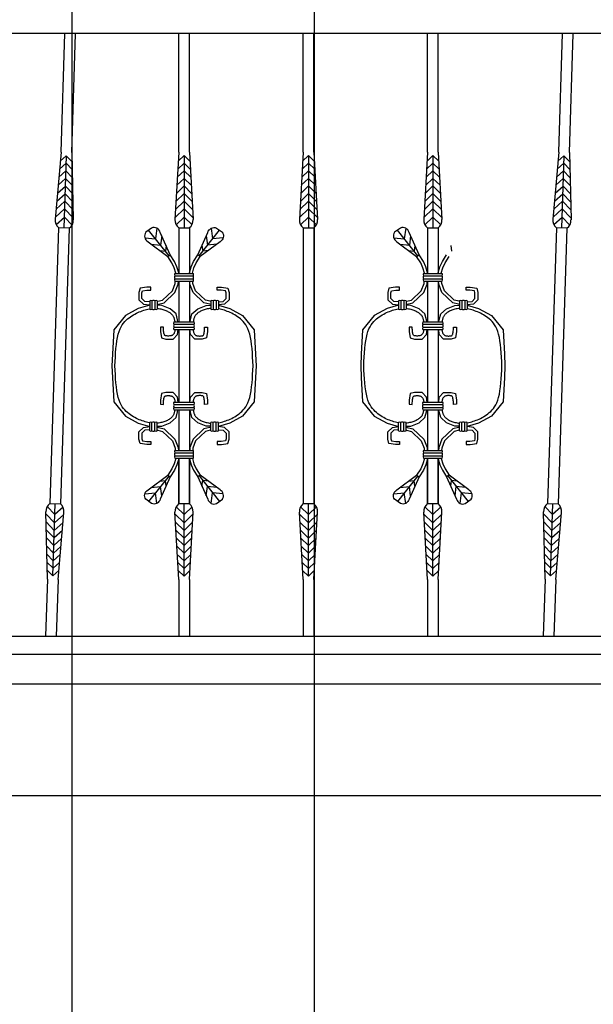
# Model space of a CAD drawing. Units: inches. Extents: x 2278 to 7495, y -71 to 1198.
# Tile 11 of 44: x 4907 to 4938, y 107 to 160. Entities that reach past the tile are written whole.
import ezdxf

# ---------------------------------------------------------------- set-up
doc = ezdxf.new("R2010")
doc.units = ezdxf.units.IN
doc.header["$MEASUREMENT"] = 0
doc.layers.add('A-ANNO-DIMS', color=2, linetype='Continuous', lineweight=18)
doc.layers.add('A-ELEV', color=7, linetype='Continuous', lineweight=25)
doc.styles.get("Standard").update_dxf_attribs({"font": 'arial.ttf'})
doc.dimstyles.get("Standard").update_dxf_attribs({"dimtxt": 6, "dimasz": 3, "dimexe": 0.18, "dimexo": 0.0625, "dimgap": 0.09, "dimtad": 0, "dimtih": 1, "dimtoh": 1, "dimdec": 0, "dimzin": 0, "dimdsep": 46, "dimlunit": 3, "dimtxsty": 'Standard', "dimblk": 'ARCHTICK', "dimcen": 0.09, "dimadec": 0, "dimazin": 0, "dimtfac": 1, "dimtdec": 0, "dimtofl": 0, "dimtmove": 0, "dimatfit": 3, "dimfxl": 1, "dimtolj": 1, "dimtzin": 0, "dimarcsym": 0})

# ---------------------------------------------------------------- blocks, each defined once
blk = doc.blocks.new('BALUSTER-ORNATE-C')
for p, q in [((3.585, 26.003), (3.585, 32.384)), ((4.155, 26.003), (4.155, 32.38)), ((3.585, 26.003), (3.383, 22.393)), ((4.155, 26.003), (4.357, 22.393)), ((3.533, 25.084), (3.87, 25.41)), ((3.557, 25.516), (3.87, 25.818)), ((3.87, 25.818), (3.87, 21.929)), ((4.182, 25.516), (3.87, 25.818)), ((4.206, 25.084), (3.87, 25.41)), ((3.509, 24.653), (3.87, 25.001)), ((4.231, 24.653), (3.87, 25.001)), ((3.485, 24.221), (3.87, 24.593)), ((4.255, 24.221), (3.87, 24.593)), ((3.461, 23.79), (3.87, 24.185)), ((4.279, 23.79), (3.87, 24.185)), ((3.412, 22.927), (3.87, 23.369)), ((3.437, 23.358), (3.87, 23.777)), ((4.303, 23.358), (3.87, 23.777)), ((4.327, 22.927), (3.87, 23.369)), ((3.388, 22.495), (3.87, 22.961)), ((4.351, 22.495), (3.87, 22.961)), ((3.441, 22.106), (3.87, 22.52)), ((4.298, 22.106), (3.87, 22.52)), ((3.063, 20.442), (1.97, 21.814)), ((2.412, 21.914), (2.338, 21.352)), ((3.585, 21.929), (3.585, 19.485)), ((4.155, 21.929), (3.585, 21.929)), ((4.155, 21.929), (4.155, 19.485)), ((4.677, 20.442), (5.769, 21.814)), ((5.328, 21.914), (5.401, 21.352)), ((1.774, 21.406), (2.338, 21.352)), ((2.678, 21.507), (2.613, 21.007)), ((5.061, 21.507), (5.127, 21.007)), ((5.966, 21.406), (5.401, 21.352)), ((2.111, 21.055), (2.613, 21.007)), ((2.562, 20.717), (2.867, 20.688)), ((2.907, 20.992), (2.867, 20.688)), ((4.833, 20.992), (4.872, 20.688)), ((5.177, 20.717), (4.872, 20.688)), ((5.629, 21.055), (5.127, 21.007)), ((3.37, 19.485), (4.37, 19.485)), ((3.37, 19.363), (4.37, 19.363)), ((3.37, 19.2), (4.37, 19.2)), ((3.37, 19.077), (4.37, 19.077)), ((3.585, 19.077), (3.585, 16.887)), ((4.155, 19.077), (4.155, 16.887)), ((2.026, 18.021), (2.026, 17.565)), ((2.148, 18.021), (2.148, 17.565)), ((2.311, 18.021), (2.311, 17.565)), ((2.433, 18.021), (2.433, 17.565)), ((5.306, 18.021), (5.306, 17.565)), ((5.428, 18.021), (5.428, 17.565)), ((5.591, 18.021), (5.591, 17.565)), ((5.714, 18.021), (5.714, 17.565)), ((3.329, 16.887), (4.411, 16.887)), ((3.329, 16.764), (4.411, 16.764)), ((3.329, 16.601), (4.411, 16.601)), ((3.329, 16.479), (4.411, 16.479)), ((3.585, 16.479), (3.585, 12.578)), ((4.155, 16.479), (4.155, 12.578)), ((3.329, 12.578), (4.411, 12.578)), ((3.329, 12.456), (4.411, 12.456)), ((3.329, 12.293), (4.411, 12.293)), ((3.329, 12.171), (4.411, 12.171)), ((3.585, 12.171), (3.585, 9.98)), ((4.155, 12.171), (4.155, 9.98)), ((2.026, 11.037), (2.026, 11.493)), ((2.148, 11.037), (2.148, 11.493)), ((2.311, 11.037), (2.311, 11.493)), ((2.433, 11.037), (2.433, 11.493)), ((5.306, 11.037), (5.306, 11.493)), ((5.428, 11.037), (5.428, 11.493)), ((5.591, 11.037), (5.591, 11.493)), ((5.714, 11.037), (5.714, 11.493)), ((3.37, 9.98), (4.37, 9.98)), ((3.37, 9.858), (4.37, 9.858)), ((3.37, 9.695), (4.37, 9.695)), ((3.37, 9.573), (4.37, 9.573)), ((3.585, 9.573), (3.585, 7.095)), ((3.585, 7.095), (3.585, 9.573)), ((4.155, 9.573), (4.155, 7.095)), ((4.155, 7.095), (4.155, 9.573)), ((3.063, 8.615), (1.97, 7.244)), ((4.677, 8.615), (5.769, 7.244)), ((2.111, 8.002), (2.613, 8.051)), ((2.562, 8.34), (2.867, 8.37)), ((2.678, 7.551), (2.613, 8.051)), ((2.907, 8.066), (2.867, 8.37)), ((4.833, 8.066), (4.872, 8.37)), ((5.177, 8.34), (4.872, 8.37)), ((5.061, 7.551), (5.127, 8.051)), ((5.629, 8.002), (5.127, 8.051)), ((1.774, 7.651), (2.338, 7.706)), ((2.412, 7.143), (2.338, 7.706)), ((5.328, 7.143), (5.401, 7.706)), ((5.966, 7.651), (5.401, 7.706)), ((3.441, 6.952), (3.87, 6.538)), ((3.585, 7.128), (4.155, 7.128)), ((3.87, 3.24), (3.87, 7.128)), ((4.298, 6.952), (3.87, 6.538)), ((3.585, 3.055), (3.383, 6.664)), ((3.388, 6.562), (3.87, 6.097)), ((4.351, 6.562), (3.87, 6.097)), ((4.155, 3.055), (4.357, 6.664)), ((3.412, 6.131), (3.87, 5.689)), ((4.327, 6.131), (3.87, 5.689)), ((3.437, 5.699), (3.87, 5.28)), ((4.303, 5.699), (3.87, 5.28)), ((3.461, 5.268), (3.87, 4.872)), ((3.485, 4.836), (3.87, 4.464)), ((4.279, 5.268), (3.87, 4.872)), ((4.255, 4.836), (3.87, 4.464)), ((3.509, 4.405), (3.87, 4.056)), ((4.231, 4.405), (3.87, 4.056)), ((3.533, 3.973), (3.87, 3.648)), ((4.206, 3.973), (3.87, 3.648)), ((3.557, 3.542), (3.87, 3.24)), ((4.182, 3.542), (3.87, 3.24)), ((3.585, 3.055), (3.585, 0)), ((4.155, 3.055), (4.155, 0))]:
    blk.add_line(p, q)
for points in [[(3.131, 20.487), (2.594, 21.696, 0.435351), (2.128, 21.929), (1.813, 21.699, 0.435351), (1.936, 21.192), (2.995, 20.398)], [(4.608, 20.487), (5.145, 21.696, -0.435351), (5.612, 21.929), (5.927, 21.699, -0.435351), (5.804, 21.192), (4.745, 20.398)], [(3.131, 8.571), (2.594, 7.362, -0.435351), (2.128, 7.128), (1.813, 7.359, -0.435351), (1.936, 7.866), (2.995, 8.66)], [(4.608, 8.571), (5.145, 7.362, 0.435351), (5.612, 7.128), (5.927, 7.359, 0.435351), (5.804, 7.866), (4.745, 8.66)]]:
    blk.add_lwpolyline(points, format="xyb", close=True)
for points in [[(3.42, 19.485), (3.421, 19.506), (3.336, 19.795), (3.216, 20.057), (2.995, 20.398)], [(3.583, 19.485), (3.585, 19.526), (3.489, 19.852), (3.359, 20.135), (3.131, 20.487)], [(4.157, 19.485), (4.155, 19.526), (4.25, 19.852), (4.38, 20.135), (4.608, 20.487)], [(4.32, 19.485), (4.319, 19.506), (4.403, 19.795), (4.523, 20.057), (4.745, 20.398)], [(2.433, 17.826), (2.492, 17.833), (2.801, 17.915), (3.385, 18.463), (3.557, 18.908), (3.565, 19.077)], [(2.433, 17.99), (2.462, 17.993), (2.719, 18.062), (3.247, 18.557), (3.396, 18.942), (3.402, 19.077)], [(5.306, 17.826), (5.247, 17.833), (4.939, 17.915), (4.355, 18.463), (4.182, 18.908), (4.175, 19.077)], [(5.306, 17.99), (5.278, 17.993), (5.02, 18.062), (4.493, 18.557), (4.344, 18.942), (4.338, 19.077)], [(2.026, 17.961), (1.767, 17.989), (1.612, 18.138), (1.612, 18.447), (1.642, 18.56), (1.879, 18.596), (2.084, 18.596), (2.084, 18.759), (1.866, 18.759), (1.512, 18.705), (1.449, 18.469), (1.449, 18.069), (1.694, 17.833), (2.026, 17.797)], [(5.714, 17.961), (5.973, 17.989), (6.128, 18.138), (6.128, 18.447), (6.098, 18.56), (5.861, 18.596), (5.656, 18.596), (5.656, 18.759), (5.873, 18.759), (6.227, 18.705), (6.291, 18.469), (6.291, 18.069), (6.046, 17.833), (5.714, 17.797)], [(2.026, 17.782), (1.412, 17.603), (0.722, 17.231), (0.095, 16.469), (0.025, 15.162), (0, 14.529), (0.025, 13.895), (0.095, 12.589), (0.722, 11.827), (1.412, 11.455), (2.026, 11.276)], [(0.163, 14.522), (0.173, 14.759), (0.184, 14.995), (0.199, 15.227), (0.217, 15.452), (0.239, 15.667), (0.267, 15.87), (0.3, 16.057), (0.34, 16.227), (0.386, 16.376), (0.438, 16.508), (0.495, 16.624), (0.557, 16.727), (0.623, 16.819), (0.692, 16.9), (0.764, 16.975), (0.839, 17.043), (0.916, 17.105), (0.993, 17.163), (1.071, 17.216), (1.15, 17.265), (1.229, 17.309), (1.309, 17.35), (1.389, 17.388), (1.469, 17.422), (1.548, 17.454), (1.627, 17.484), (1.705, 17.51), (1.782, 17.533), (1.858, 17.553), (1.933, 17.571), (2.007, 17.585), (2.026, 17.587)], [(3.541, 16.887), (3.527, 17.004), (3.446, 17.313), (3.128, 17.594), (2.683, 17.766), (2.433, 17.777)], [(2.433, 17.606), (2.499, 17.6), (2.563, 17.592), (2.624, 17.582), (2.683, 17.57), (2.739, 17.556), (2.792, 17.54), (2.842, 17.522), (2.891, 17.503), (2.937, 17.482), (2.981, 17.46), (3.023, 17.436), (3.064, 17.41), (3.102, 17.384), (3.138, 17.357), (3.171, 17.329), (3.201, 17.301), (3.228, 17.272), (3.251, 17.244), (3.271, 17.217), (3.288, 17.19), (3.303, 17.162), (3.316, 17.134), (3.327, 17.104), (3.337, 17.072), (3.345, 17.038), (3.354, 17.001), (3.361, 16.962), (3.368, 16.922), (3.374, 16.887)], [(4.198, 16.887), (4.212, 17.004), (4.294, 17.313), (4.612, 17.594), (5.057, 17.766), (5.306, 17.777)], [(5.306, 17.606), (5.241, 17.6), (5.177, 17.592), (5.115, 17.582), (5.057, 17.57), (5.001, 17.556), (4.948, 17.54), (4.897, 17.522), (4.849, 17.503), (4.803, 17.482), (4.759, 17.46), (4.716, 17.436), (4.676, 17.41), (4.638, 17.384), (4.602, 17.357), (4.569, 17.329), (4.539, 17.301), (4.512, 17.272), (4.488, 17.244), (4.468, 17.217), (4.451, 17.19), (4.437, 17.162), (4.424, 17.134), (4.413, 17.104), (4.403, 17.072), (4.394, 17.038), (4.386, 17.001), (4.379, 16.962), (4.371, 16.922), (4.366, 16.887)], [(5.714, 17.782), (6.328, 17.603), (7.018, 17.231), (7.644, 16.469), (7.715, 15.162), (7.74, 14.529), (7.715, 13.895), (7.644, 12.589), (7.018, 11.827), (6.328, 11.455), (5.714, 11.276)], [(7.577, 14.522), (7.567, 14.759), (7.555, 14.995), (7.541, 15.227), (7.523, 15.452), (7.501, 15.667), (7.473, 15.87), (7.44, 16.057), (7.4, 16.227), (7.354, 16.376), (7.302, 16.508), (7.244, 16.624), (7.183, 16.727), (7.117, 16.819), (7.048, 16.9), (6.976, 16.975), (6.901, 17.043), (6.824, 17.105), (6.747, 17.163), (6.668, 17.216), (6.59, 17.265), (6.51, 17.309), (6.431, 17.35), (6.351, 17.388), (6.271, 17.422), (6.191, 17.454), (6.113, 17.484), (6.035, 17.51), (5.958, 17.533), (5.882, 17.553), (5.807, 17.571), (5.733, 17.585), (5.714, 17.587)], [(3.388, 16.479), (3.383, 16.441), (3.376, 16.401), (3.368, 16.364), (3.357, 16.329), (3.346, 16.299), (3.333, 16.271), (3.318, 16.247), (3.303, 16.225), (3.286, 16.207), (3.268, 16.19), (3.249, 16.176), (3.228, 16.164), (3.205, 16.154), (3.179, 16.145), (3.149, 16.138), (3.116, 16.133), (3.081, 16.13), (3.045, 16.129), (3.007, 16.129), (2.971, 16.131), (2.936, 16.134), (2.905, 16.137), (2.88, 16.142), (2.863, 16.146), (2.852, 16.151), (2.845, 16.154), (2.84, 16.159), (2.834, 16.166), (2.825, 16.18), (2.814, 16.203), (2.803, 16.237), (2.792, 16.28), (2.783, 16.331), (2.775, 16.388), (2.769, 16.452), (2.766, 16.522), (2.764, 16.599), (2.601, 16.596), (2.601, 16.378), (2.656, 16.024), (2.892, 15.961), (3.291, 15.961), (3.527, 16.206), (3.557, 16.479)], [(4.352, 16.479), (4.357, 16.441), (4.364, 16.401), (4.372, 16.364), (4.382, 16.329), (4.394, 16.299), (4.407, 16.271), (4.421, 16.247), (4.437, 16.225), (4.454, 16.207), (4.472, 16.19), (4.491, 16.176), (4.512, 16.164), (4.534, 16.154), (4.56, 16.145), (4.59, 16.138), (4.623, 16.133), (4.659, 16.13), (4.695, 16.129), (4.732, 16.129), (4.769, 16.131), (4.804, 16.134), (4.835, 16.137), (4.86, 16.142), (4.877, 16.146), (4.888, 16.151), (4.894, 16.154), (4.899, 16.159), (4.906, 16.166), (4.914, 16.18), (4.925, 16.203), (4.937, 16.237), (4.948, 16.28), (4.957, 16.331), (4.965, 16.388), (4.971, 16.452), (4.974, 16.522), (4.975, 16.599), (5.138, 16.596), (5.138, 16.378), (5.084, 16.024), (4.848, 15.961), (4.448, 15.961), (4.212, 16.206), (4.182, 16.479)], [(2.026, 11.47), (2.007, 11.473), (1.933, 11.487), (1.858, 11.504), (1.782, 11.524), (1.705, 11.548), (1.627, 11.574), (1.548, 11.603), (1.469, 11.635), (1.389, 11.67), (1.309, 11.708), (1.229, 11.748), (1.15, 11.793), (1.071, 11.841), (0.993, 11.894), (0.916, 11.952), (0.839, 12.015), (0.764, 12.083), (0.692, 12.157), (0.623, 12.239), (0.557, 12.33), (0.495, 12.433), (0.438, 12.549), (0.386, 12.681), (0.34, 12.831), (0.3, 13), (0.267, 13.188), (0.239, 13.391), (0.217, 13.606), (0.199, 13.831), (0.184, 14.062), (0.173, 14.298), (0.163, 14.536)], [(5.714, 11.47), (5.733, 11.473), (5.807, 11.487), (5.882, 11.504), (5.958, 11.524), (6.035, 11.548), (6.113, 11.574), (6.191, 11.603), (6.271, 11.635), (6.351, 11.67), (6.431, 11.708), (6.51, 11.748), (6.59, 11.793), (6.668, 11.841), (6.747, 11.894), (6.824, 11.952), (6.901, 12.015), (6.976, 12.083), (7.048, 12.157), (7.117, 12.239), (7.183, 12.33), (7.244, 12.433), (7.302, 12.549), (7.354, 12.681), (7.4, 12.831), (7.44, 13), (7.473, 13.188), (7.501, 13.391), (7.523, 13.606), (7.541, 13.831), (7.555, 14.062), (7.567, 14.298), (7.577, 14.536)], [(3.557, 12.578), (3.527, 12.852), (3.291, 13.097), (2.892, 13.097), (2.656, 13.033), (2.601, 12.679), (2.601, 12.462), (2.764, 12.459), (2.766, 12.536), (2.769, 12.605), (2.775, 12.669), (2.783, 12.727), (2.792, 12.778), (2.803, 12.82), (2.814, 12.854), (2.825, 12.878), (2.834, 12.892), (2.84, 12.899), (2.845, 12.903), (2.852, 12.907), (2.863, 12.911), (2.88, 12.916), (2.905, 12.92), (2.936, 12.924), (2.971, 12.927), (3.007, 12.929), (3.045, 12.929), (3.081, 12.928), (3.116, 12.924), (3.149, 12.919), (3.179, 12.912), (3.205, 12.904), (3.228, 12.893), (3.249, 12.881), (3.268, 12.867), (3.286, 12.851), (3.303, 12.832), (3.318, 12.811), (3.333, 12.786), (3.346, 12.759), (3.357, 12.728), (3.368, 12.694), (3.376, 12.656), (3.383, 12.616), (3.388, 12.578)], [(4.182, 12.578), (4.212, 12.852), (4.448, 13.097), (4.848, 13.097), (5.084, 13.033), (5.138, 12.679), (5.138, 12.462), (4.975, 12.459), (4.974, 12.536), (4.971, 12.605), (4.965, 12.669), (4.957, 12.727), (4.948, 12.778), (4.937, 12.82), (4.925, 12.854), (4.914, 12.878), (4.906, 12.892), (4.899, 12.899), (4.894, 12.903), (4.888, 12.907), (4.877, 12.911), (4.86, 12.916), (4.835, 12.92), (4.804, 12.924), (4.769, 12.927), (4.732, 12.929), (4.695, 12.929), (4.659, 12.928), (4.623, 12.924), (4.59, 12.919), (4.56, 12.912), (4.534, 12.904), (4.512, 12.893), (4.491, 12.881), (4.472, 12.867), (4.454, 12.851), (4.437, 12.832), (4.421, 12.811), (4.407, 12.786), (4.394, 12.759), (4.382, 12.728), (4.372, 12.694), (4.364, 12.656), (4.357, 12.616), (4.352, 12.578)], [(3.374, 12.171), (3.368, 12.136), (3.361, 12.095), (3.354, 12.056), (3.345, 12.02), (3.337, 11.986), (3.327, 11.954), (3.316, 11.924), (3.303, 11.895), (3.288, 11.868), (3.271, 11.841), (3.251, 11.813), (3.228, 11.785), (3.201, 11.757), (3.171, 11.729), (3.138, 11.701), (3.102, 11.673), (3.064, 11.647), (3.023, 11.622), (2.981, 11.598), (2.937, 11.576), (2.891, 11.555), (2.842, 11.535), (2.792, 11.518), (2.739, 11.502), (2.683, 11.488), (2.624, 11.476), (2.563, 11.465), (2.499, 11.457), (2.433, 11.451)], [(2.433, 11.28), (2.683, 11.291), (3.128, 11.464), (3.446, 11.745), (3.527, 12.053), (3.541, 12.171)], [(5.306, 11.28), (5.057, 11.291), (4.612, 11.464), (4.294, 11.745), (4.212, 12.053), (4.198, 12.171)], [(4.366, 12.171), (4.371, 12.136), (4.379, 12.095), (4.386, 12.056), (4.394, 12.02), (4.403, 11.986), (4.413, 11.954), (4.424, 11.924), (4.437, 11.895), (4.451, 11.868), (4.468, 11.841), (4.488, 11.813), (4.512, 11.785), (4.539, 11.757), (4.569, 11.729), (4.602, 11.701), (4.638, 11.673), (4.676, 11.647), (4.716, 11.622), (4.759, 11.598), (4.803, 11.576), (4.849, 11.555), (4.897, 11.535), (4.948, 11.518), (5.001, 11.502), (5.057, 11.488), (5.115, 11.476), (5.177, 11.465), (5.241, 11.457), (5.306, 11.451)], [(2.026, 11.097), (1.767, 11.069), (1.612, 10.919), (1.612, 10.611), (1.642, 10.498), (1.879, 10.461), (2.084, 10.461), (2.084, 10.298), (1.866, 10.298), (1.512, 10.353), (1.449, 10.589), (1.449, 10.988), (1.694, 11.225), (2.026, 11.261)], [(2.433, 11.232), (2.492, 11.225), (2.801, 11.143), (3.385, 10.594), (3.557, 10.149), (3.565, 9.98)], [(5.306, 11.232), (5.247, 11.225), (4.939, 11.143), (4.355, 10.594), (4.182, 10.149), (4.175, 9.98)], [(5.714, 11.097), (5.973, 11.069), (6.128, 10.919), (6.128, 10.611), (6.098, 10.498), (5.861, 10.461), (5.656, 10.461), (5.656, 10.298), (5.873, 10.298), (6.227, 10.353), (6.291, 10.589), (6.291, 10.988), (6.046, 11.225), (5.714, 11.261)], [(2.433, 11.067), (2.462, 11.064), (2.719, 10.996), (3.247, 10.501), (3.396, 10.115), (3.402, 9.98)], [(5.306, 11.067), (5.278, 11.064), (5.02, 10.996), (4.493, 10.501), (4.344, 10.115), (4.338, 9.98)], [(3.42, 9.573), (3.421, 9.552), (3.336, 9.262), (3.216, 9.001), (2.995, 8.66)], [(3.583, 9.573), (3.585, 9.532), (3.489, 9.205), (3.359, 8.922), (3.131, 8.571)], [(4.157, 9.573), (4.155, 9.532), (4.25, 9.205), (4.38, 8.922), (4.608, 8.571)], [(4.32, 9.573), (4.319, 9.552), (4.403, 9.262), (4.523, 9.001), (4.745, 8.66)]]:
    blk.add_lwpolyline(points)
for centre, radius, start, end in [((3.929, 22.355), 0.547, 176.0178, 231.0717), ((3.811, 22.355), 0.547, 308.9283, 3.9822), ((3.475, 19.424), 0.121, 149.7768, 210.2232), ((3.563, 19.281), 0.209, 157.1017, 202.8983), ((3.475, 19.139), 0.121, 149.7768, 210.2232), ((4.265, 19.424), 0.121, 329.7768, 30.2232), ((4.177, 19.281), 0.209, 337.1017, 22.8983), ((4.265, 19.139), 0.121, 329.7768, 30.2232), ((2.087, 17.916), 0.121, 59.7768, 120.2232), ((2.23, 17.828), 0.209, 67.1017, 112.8983), ((2.372, 17.916), 0.121, 59.7768, 120.2232), ((5.367, 17.916), 0.121, 59.7768, 120.2232), ((5.51, 17.828), 0.209, 67.1017, 112.8983), ((5.653, 17.916), 0.121, 59.7768, 120.2232), ((2.087, 17.67), 0.121, 239.7768, 300.2232), ((2.23, 17.758), 0.209, 247.1017, 292.8983), ((2.372, 17.67), 0.121, 239.7768, 300.2232), ((5.367, 17.67), 0.121, 239.7768, 300.2232), ((5.51, 17.758), 0.209, 247.1017, 292.8983), ((5.653, 17.67), 0.121, 239.7768, 300.2232), ((3.434, 16.825), 0.121, 149.7768, 210.2232), ((3.522, 16.683), 0.209, 157.1017, 202.8983), ((3.434, 16.54), 0.121, 149.7768, 210.2232), ((4.306, 16.825), 0.121, 329.7768, 30.2232), ((4.218, 16.683), 0.209, 337.1017, 22.8983), ((4.306, 16.54), 0.121, 329.7768, 30.2232), ((3.434, 12.517), 0.121, 149.7768, 210.2232), ((3.522, 12.375), 0.209, 157.1017, 202.8983), ((3.434, 12.232), 0.121, 149.7768, 210.2232), ((4.306, 12.517), 0.121, 329.7768, 30.2232), ((4.218, 12.375), 0.209, 337.1017, 22.8983), ((4.306, 12.232), 0.121, 329.7768, 30.2232), ((2.087, 11.388), 0.121, 59.7768, 120.2232), ((2.23, 11.3), 0.209, 67.1017, 112.8983), ((2.372, 11.388), 0.121, 59.7768, 120.2232), ((5.367, 11.388), 0.121, 59.7768, 120.2232), ((5.51, 11.3), 0.209, 67.1017, 112.8983), ((5.653, 11.388), 0.121, 59.7768, 120.2232), ((2.087, 11.142), 0.121, 239.7768, 300.2232), ((2.23, 11.23), 0.209, 247.1017, 292.8983), ((2.372, 11.142), 0.121, 239.7768, 300.2232), ((5.367, 11.142), 0.121, 239.7768, 300.2232), ((5.51, 11.23), 0.209, 247.1017, 292.8983), ((5.653, 11.142), 0.121, 239.7768, 300.2232), ((3.475, 9.919), 0.121, 149.7768, 210.2232), ((3.563, 9.776), 0.209, 157.1017, 202.8983), ((3.475, 9.634), 0.121, 149.7768, 210.2232), ((4.265, 9.919), 0.121, 329.7768, 30.2232), ((4.177, 9.776), 0.209, 337.1017, 22.8983), ((4.265, 9.634), 0.121, 329.7768, 30.2232), ((3.929, 6.703), 0.547, 128.9283, 183.9822), ((3.811, 6.703), 0.547, 356.0178, 51.0717)]:
    blk.add_arc(centre, radius, start, end)
blk = doc.blocks.new('RAIL-BAR-A')
for p, q in [((0.202, 26.003), (0.202, 32.38)), ((0.773, 26.003), (0.773, 32.38)), ((0.202, 26.003), (0, 22.393)), ((0.773, 26.003), (0.975, 22.393)), ((0.151, 25.084), (0.488, 25.41)), ((0.175, 25.516), (0.488, 25.818)), ((0.488, 25.818), (0.488, 21.929)), ((0.8, 25.516), (0.488, 25.818)), ((0.824, 25.084), (0.488, 25.41)), ((0.127, 24.653), (0.488, 25.001)), ((0.848, 24.653), (0.488, 25.001)), ((0.103, 24.221), (0.488, 24.593)), ((0.873, 24.221), (0.488, 24.593)), ((0.079, 23.79), (0.488, 24.185)), ((0.897, 23.79), (0.488, 24.185)), ((0.03, 22.927), (0.488, 23.369)), ((0.054, 23.358), (0.488, 23.777)), ((0.921, 23.358), (0.488, 23.777)), ((0.945, 22.927), (0.488, 23.369)), ((0.006, 22.495), (0.488, 22.961)), ((0.969, 22.495), (0.488, 22.961)), ((0.059, 22.106), (0.488, 22.52)), ((0.916, 22.106), (0.488, 22.52)), ((0.202, 21.929), (0.202, 7.128)), ((0.773, 21.929), (0.202, 21.929)), ((0.773, 21.929), (0.773, 7.128)), ((0.059, 6.952), (0.488, 6.538)), ((0.202, 7.128), (0.773, 7.128)), ((0.488, 3.24), (0.488, 7.128)), ((0.916, 6.952), (0.488, 6.538)), ((0.202, 3.055), (0, 6.664)), ((0.006, 6.562), (0.488, 6.097)), ((0.969, 6.562), (0.488, 6.097)), ((0.773, 3.055), (0.975, 6.664)), ((0.03, 6.131), (0.488, 5.689)), ((0.945, 6.131), (0.488, 5.689)), ((0.054, 5.699), (0.488, 5.28)), ((0.921, 5.699), (0.488, 5.28)), ((0.079, 5.268), (0.488, 4.872)), ((0.103, 4.836), (0.488, 4.464)), ((0.897, 5.268), (0.488, 4.872)), ((0.873, 4.836), (0.488, 4.464)), ((0.127, 4.405), (0.488, 4.056)), ((0.848, 4.405), (0.488, 4.056)), ((0.151, 3.973), (0.488, 3.648)), ((0.824, 3.973), (0.488, 3.648)), ((0.175, 3.542), (0.488, 3.24)), ((0.8, 3.542), (0.488, 3.24)), ((0.202, 3.055), (0.202, 0)), ((0.773, 3.055), (0.773, 0))]:
    blk.add_line(p, q)
for centre, start, end in [((0.546, 22.355), 176.0178, 231.0717), ((0.429, 22.355), 308.9283, 3.9822), ((0.546, 6.703), 128.9283, 183.9822), ((0.429, 6.703), 356.0178, 51.0717)]:
    blk.add_arc(centre, 0.547, start, end)
blk = doc.blocks.new('RAIL-BAR-C')
for p, q in [((0.203, 26.003), (0.203, 32.38)), ((0.773, 32.38), (0.203, 32.38)), ((0.773, 26.003), (0.773, 32.38)), ((0.203, 26.003), (0, 22.393)), ((0.773, 26.003), (0.975, 22.393)), ((0.151, 25.084), (0.488, 25.41)), ((0.175, 25.516), (0.488, 25.818)), ((0.488, 25.818), (0.488, 21.929)), ((0.8, 25.516), (0.488, 25.818)), ((0.824, 25.084), (0.488, 25.41)), ((0.127, 24.653), (0.488, 25.001)), ((0.848, 24.653), (0.488, 25.001)), ((0.103, 24.221), (0.488, 24.593)), ((0.873, 24.221), (0.488, 24.593)), ((0.079, 23.79), (0.488, 24.185)), ((0.897, 23.79), (0.488, 24.185)), ((0.03, 22.927), (0.488, 23.369)), ((0.054, 23.358), (0.488, 23.777)), ((0.921, 23.358), (0.488, 23.777)), ((0.945, 22.927), (0.488, 23.369)), ((0.006, 22.495), (0.488, 22.961)), ((0.969, 22.495), (0.488, 22.961)), ((0.059, 22.106), (0.488, 22.52)), ((0.916, 22.106), (0.488, 22.52)), ((0.203, 21.929), (0.203, 7.128)), ((0.773, 21.929), (0.203, 21.929)), ((0.773, 21.929), (0.773, 7.128)), ((0.059, 6.952), (0.488, 6.538)), ((0.203, 7.128), (0.773, 7.128)), ((0.488, 3.24), (0.488, 7.128)), ((0.916, 6.952), (0.488, 6.538)), ((0.203, 3.055), (0, 6.664)), ((0.006, 6.562), (0.488, 6.097)), ((0.969, 6.562), (0.488, 6.097)), ((0.773, 3.055), (0.975, 6.664)), ((0.03, 6.131), (0.488, 5.689)), ((0.945, 6.131), (0.488, 5.689)), ((0.054, 5.699), (0.488, 5.28)), ((0.921, 5.699), (0.488, 5.28)), ((0.079, 5.268), (0.488, 4.872)), ((0.103, 4.836), (0.488, 4.464)), ((0.897, 5.268), (0.488, 4.872)), ((0.873, 4.836), (0.488, 4.464)), ((0.127, 4.405), (0.488, 4.056)), ((0.848, 4.405), (0.488, 4.056)), ((0.151, 3.973), (0.488, 3.648)), ((0.824, 3.973), (0.488, 3.648)), ((0.175, 3.542), (0.488, 3.24)), ((0.8, 3.542), (0.488, 3.24)), ((0.203, 3.055), (0.203, 0)), ((0.773, 3.055), (0.773, 0))]:
    blk.add_line(p, q)
for centre, start, end in [((0.547, 22.355), 176.0178, 231.0717), ((0.429, 22.355), 308.9283, 3.9822), ((0.547, 6.703), 128.9283, 183.9822), ((0.429, 6.703), 356.0178, 51.0717)]:
    blk.add_arc(centre, 0.547, start, end)
blk = doc.blocks.new('_ArchTick')
at = {"color": 0, "linetype": 'ByBlock', "const_width": 0.15}
blk.add_lwpolyline([(-0.5, -0.5), (0.5, 0.5)], dxfattribs=at)
blk = doc.blocks.new('*D123')
at = {"layer": 'A-ANNO-DIMS', "color": 0, "lineweight": -2, "transparency": 16777216}
for p, q in [((4736.95, 340.157), (4736.95, -23.427)), ((5145.676, -1.81), (5145.676, -23.427)), ((4736.95, -23.247), (4923.929, -23.247)), ((5145.676, -23.247), (4958.697, -23.247))]:
    blk.add_line(p, q, dxfattribs=at)
at = {"layer": 'Defpoints', "color": 0, "transparency": 16777216}
for p in [(4736.95, 340.219), (5145.676, -1.747), (5145.676, -23.247)]:
    blk.add_point(p, dxfattribs=at)
at = {"layer": 'A-ANNO-DIMS', "color": 0, "lineweight": -2, "transparency": 16777216, "xscale": 3, "yscale": 3, "zscale": 3, "rotation": 180}
blk.add_blockref('_ArchTick', (4736.95, -23.247), dxfattribs=at)
at = {"layer": 'A-ANNO-DIMS', "color": 0, "lineweight": -2, "transparency": 16777216, "xscale": 3, "yscale": 3, "zscale": 3}
blk.add_blockref('_ArchTick', (5145.676, -23.247), dxfattribs=at)
at = {"layer": 'A-ANNO-DIMS', "color": 0, "transparency": 16777216, "insert": (4941.313, -23.247), "char_height": 6, "attachment_point": 5}
blk.add_mtext('\\A1;34\'-0 1/2"', dxfattribs=at)
blk = doc.blocks.new('*D127')
at = {"layer": 'A-ANNO-DIMS', "color": 0, "lineweight": -2, "transparency": 16777216}
for p, q in [((4874.676, 99.315), (4874.676, 361.899)), ((4874.676, 361.719), (4881.729, 361.719)), ((4909.676, 361.719), (4902.623, 361.719)), ((4909.676, 99.315), (4909.676, 361.899))]:
    blk.add_line(p, q, dxfattribs=at)
at = {"layer": 'Defpoints', "color": 0, "transparency": 16777216}
for p in [(4909.676, 361.719), (4874.676, 99.253), (4909.676, 99.253)]:
    blk.add_point(p, dxfattribs=at)
at = {"layer": 'A-ANNO-DIMS', "color": 0, "lineweight": -2, "transparency": 16777216, "xscale": 3, "yscale": 3, "zscale": 3, "rotation": 180}
blk.add_blockref('_ArchTick', (4874.676, 361.719), dxfattribs=at)
at = {"layer": 'A-ANNO-DIMS', "color": 0, "lineweight": -2, "transparency": 16777216, "xscale": 3, "yscale": 3, "zscale": 3}
blk.add_blockref('_ArchTick', (4909.676, 361.719), dxfattribs=at)
at = {"layer": 'A-ANNO-DIMS', "color": 0, "transparency": 16777216, "insert": (4892.176, 361.719), "char_height": 6, "attachment_point": 5}
blk.add_mtext('\\A1;2\'-11"', dxfattribs=at)
blk = doc.blocks.new('*D128')
at = {"layer": 'A-ANNO-DIMS', "color": 0, "lineweight": -2, "transparency": 16777216}
for p, q in [((4909.676, 99.315), (4909.676, 361.899)), ((4909.676, 361.719), (4932.111, 361.719)), ((4970.676, 361.719), (4948.241, 361.719)), ((4970.676, 60.779), (4970.676, 361.899))]:
    blk.add_line(p, q, dxfattribs=at)
at = {"layer": 'Defpoints', "color": 0, "transparency": 16777216}
for p in [(4970.676, 361.719), (4909.676, 99.253), (4970.676, 60.717)]:
    blk.add_point(p, dxfattribs=at)
at = {"layer": 'A-ANNO-DIMS', "color": 0, "lineweight": -2, "transparency": 16777216, "xscale": 3, "yscale": 3, "zscale": 3, "rotation": 180}
blk.add_blockref('_ArchTick', (4909.676, 361.719), dxfattribs=at)
at = {"layer": 'A-ANNO-DIMS', "color": 0, "lineweight": -2, "transparency": 16777216, "xscale": 3, "yscale": 3, "zscale": 3}
blk.add_blockref('_ArchTick', (4970.676, 361.719), dxfattribs=at)
at = {"layer": 'A-ANNO-DIMS', "color": 0, "transparency": 16777216, "insert": (4940.176, 361.719), "char_height": 6, "attachment_point": 5}
blk.add_mtext('\\A1;5\'-1"', dxfattribs=at)

msp = doc.modelspace()

# ---------------------------------------------------------------- linework, layer by layer
at = {"layer": 'A-ELEV'}
for p, q in [((4922.676, 66.655), (4922.676, 244.253)), ((4969.039, 159.179), (4875.673, 159.179)), ((4928.751, 152.802), (4928.751, 159.183)), ((4929.322, 152.802), (4929.322, 159.179)), ((4928.751, 152.802), (4928.549, 149.192)), ((4928.724, 152.315), (4929.037, 152.617)), ((4929.037, 152.617), (4929.037, 148.728)), ((4929.349, 152.315), (4929.037, 152.617)), ((4929.322, 152.802), (4929.524, 149.192)), ((4928.676, 151.452), (4929.037, 151.8)), ((4928.7, 151.883), (4929.037, 152.209)), ((4929.373, 151.883), (4929.037, 152.209)), ((4929.397, 151.452), (4929.037, 151.8)), ((4928.652, 151.02), (4929.037, 151.392)), ((4929.421, 151.02), (4929.037, 151.392)), ((4928.627, 150.589), (4929.037, 150.984)), ((4929.446, 150.589), (4929.037, 150.984)), ((4928.579, 149.726), (4929.037, 150.168)), ((4928.603, 150.157), (4929.037, 150.576)), ((4929.47, 150.157), (4929.037, 150.576)), ((4929.494, 149.726), (4929.037, 150.168)), ((4928.555, 149.294), (4929.037, 149.76)), ((4929.518, 149.294), (4929.037, 149.76)), ((4928.608, 148.905), (4929.037, 149.319)), ((4929.465, 148.905), (4929.037, 149.319)), ((4928.23, 147.241), (4927.137, 148.613)), ((4927.578, 148.713), (4927.505, 148.151)), ((4928.751, 148.728), (4928.751, 146.284)), ((4929.322, 148.728), (4928.751, 148.728)), ((4929.322, 148.728), (4929.322, 146.284)), ((4926.941, 148.205), (4927.505, 148.151)), ((4927.845, 148.306), (4927.78, 147.806)), ((4927.278, 147.854), (4927.78, 147.806)), ((4928.074, 147.791), (4928.034, 147.487)), ((4929.999, 147.791), (4930.039, 147.487)), ((4927.729, 147.516), (4928.034, 147.487)), ((4928.537, 146.284), (4929.537, 146.284)), ((4928.537, 146.162), (4929.537, 146.162)), ((4928.537, 145.999), (4929.537, 145.999)), ((4928.537, 145.876), (4929.537, 145.876)), ((4928.751, 145.876), (4928.751, 143.686)), ((4929.322, 145.876), (4929.322, 143.686)), ((4927.193, 144.82), (4927.193, 144.364)), ((4927.315, 144.82), (4927.315, 144.364)), ((4927.478, 144.82), (4927.478, 144.364)), ((4927.6, 144.82), (4927.6, 144.364)), ((4930.473, 144.82), (4930.473, 144.364)), ((4930.595, 144.82), (4930.595, 144.364)), ((4930.758, 144.82), (4930.758, 144.364)), ((4930.88, 144.82), (4930.88, 144.364)), ((4928.496, 143.686), (4929.577, 143.686)), ((4928.496, 143.563), (4929.577, 143.563)), ((4928.496, 143.4), (4929.577, 143.4)), ((4928.496, 143.278), (4929.577, 143.278)), ((4928.751, 143.278), (4928.751, 139.377)), ((4929.322, 143.278), (4929.322, 139.377)), ((4928.496, 139.377), (4929.577, 139.377)), ((4928.496, 139.255), (4929.577, 139.255)), ((4928.496, 139.092), (4929.577, 139.092)), ((4928.496, 138.97), (4929.577, 138.97)), ((4928.751, 138.97), (4928.751, 136.779)), ((4929.322, 138.97), (4929.322, 136.779)), ((4927.193, 137.836), (4927.193, 138.292)), ((4927.315, 137.836), (4927.315, 138.292)), ((4927.478, 137.836), (4927.478, 138.292)), ((4927.6, 137.836), (4927.6, 138.292)), ((4930.473, 137.836), (4930.473, 138.292)), ((4930.595, 137.836), (4930.595, 138.292)), ((4930.758, 137.836), (4930.758, 138.292)), ((4930.88, 137.836), (4930.88, 138.292)), ((4928.537, 136.779), (4929.537, 136.779)), ((4928.537, 136.657), (4929.537, 136.657)), ((4928.537, 136.494), (4929.537, 136.494)), ((4928.537, 136.372), (4929.537, 136.372)), ((4928.751, 136.372), (4928.751, 133.894)), ((4928.751, 133.894), (4928.751, 136.372)), ((4929.322, 136.372), (4929.322, 133.894)), ((4929.322, 133.894), (4929.322, 136.372)), ((4928.23, 135.414), (4927.137, 134.043)), ((4929.843, 135.414), (4930.936, 134.043)), ((4927.278, 134.801), (4927.78, 134.85)), ((4927.729, 135.139), (4928.034, 135.169)), ((4927.845, 134.35), (4927.78, 134.85)), ((4928.074, 134.865), (4928.034, 135.169)), ((4929.999, 134.865), (4930.039, 135.169)), ((4930.344, 135.139), (4930.039, 135.169)), ((4930.228, 134.35), (4930.293, 134.85)), ((4930.795, 134.801), (4930.293, 134.85)), ((4926.941, 134.45), (4927.505, 134.505)), ((4927.578, 133.942), (4927.505, 134.505)), ((4930.495, 133.942), (4930.568, 134.505)), ((4931.132, 134.45), (4930.568, 134.505)), ((4928.751, 133.927), (4929.322, 133.927)), ((4929.037, 130.039), (4929.037, 133.927)), ((4928.751, 129.854), (4928.549, 133.463)), ((4928.555, 133.361), (4929.037, 132.896)), ((4928.608, 133.751), (4929.037, 133.337)), ((4929.465, 133.751), (4929.037, 133.337)), ((4929.518, 133.361), (4929.037, 132.896)), ((4929.322, 129.854), (4929.524, 133.463)), ((4928.579, 132.93), (4929.037, 132.488)), ((4929.494, 132.93), (4929.037, 132.488)), ((4928.603, 132.498), (4929.037, 132.079)), ((4929.47, 132.498), (4929.037, 132.079)), ((4928.627, 132.067), (4929.037, 131.671)), ((4929.446, 132.067), (4929.037, 131.671)), ((4928.652, 131.635), (4929.037, 131.263)), ((4928.676, 131.204), (4929.037, 130.855)), ((4929.421, 131.635), (4929.037, 131.263)), ((4929.397, 131.204), (4929.037, 130.855)), ((4928.7, 130.772), (4929.037, 130.447)), ((4929.373, 130.772), (4929.037, 130.447)), ((4928.724, 130.341), (4929.037, 130.039)), ((4929.349, 130.341), (4929.037, 130.039)), ((4928.751, 129.854), (4928.751, 126.799)), ((4929.322, 129.854), (4929.322, 126.799)), ((4969.039, 126.799), (4875.673, 126.799)), ((4969.039, 125.821), (4875.673, 125.821)), ((4874.676, 124.253), (5145.676, 124.253)), ((4874.676, 118.253), (5145.676, 118.253))]:
    msp.add_line(p, q, dxfattribs=at)
for points in [[(4928.298, 147.286), (4927.761, 148.495, 0.435351), (4927.294, 148.728), (4926.98, 148.498, 0.435351), (4927.103, 147.991), (4928.161, 147.197)], [(4928.298, 135.37), (4927.761, 134.161, -0.435351), (4927.294, 133.927), (4926.98, 134.158, -0.435351), (4927.103, 134.665), (4928.161, 135.459)], [(4929.775, 135.37), (4930.312, 134.161, 0.435351), (4930.779, 133.927), (4931.093, 134.158, 0.435351), (4930.97, 134.665), (4929.912, 135.459)]]:
    msp.add_lwpolyline(points, format="xyb", close=True, dxfattribs=at)
for points in [[(4928.587, 146.284), (4928.587, 146.305), (4928.503, 146.594), (4928.383, 146.856), (4928.161, 147.197)], [(4928.75, 146.284), (4928.751, 146.325), (4928.656, 146.651), (4928.526, 146.934), (4928.298, 147.286)], [(4929.323, 146.284), (4929.322, 146.325), (4929.417, 146.651), (4929.547, 146.934), (4929.775, 147.286)], [(4929.487, 146.284), (4929.486, 146.305), (4929.57, 146.594), (4929.69, 146.856), (4929.912, 147.197)], [(4927.193, 144.76), (4926.934, 144.788), (4926.779, 144.937), (4926.779, 145.246), (4926.809, 145.359), (4927.045, 145.395), (4927.251, 145.395), (4927.251, 145.558), (4927.033, 145.558), (4926.679, 145.504), (4926.616, 145.268), (4926.616, 144.868), (4926.861, 144.632), (4927.193, 144.596)], [(4927.6, 144.625), (4927.659, 144.632), (4927.967, 144.714), (4928.552, 145.262), (4928.724, 145.707), (4928.732, 145.876)], [(4927.6, 144.789), (4927.628, 144.792), (4927.886, 144.861), (4928.413, 145.356), (4928.563, 145.741), (4928.569, 145.876)], [(4930.473, 144.625), (4930.414, 144.632), (4930.106, 144.714), (4929.521, 145.262), (4929.349, 145.707), (4929.341, 145.876)], [(4930.473, 144.789), (4930.445, 144.792), (4930.187, 144.861), (4929.66, 145.356), (4929.511, 145.741), (4929.505, 145.876)], [(4930.88, 144.76), (4931.14, 144.788), (4931.295, 144.937), (4931.295, 145.246), (4931.264, 145.359), (4931.028, 145.395), (4930.822, 145.395), (4930.822, 145.558), (4931.04, 145.558), (4931.394, 145.504), (4931.457, 145.268), (4931.457, 144.868), (4931.213, 144.632), (4930.88, 144.596)], [(4927.193, 144.581), (4926.579, 144.402), (4925.889, 144.03), (4925.262, 143.268), (4925.191, 141.961), (4925.167, 141.328), (4925.191, 140.694), (4925.262, 139.388), (4925.889, 138.626), (4926.579, 138.254), (4927.193, 138.075)], [(4925.33, 141.321), (4925.339, 141.558), (4925.351, 141.794), (4925.366, 142.026), (4925.384, 142.251), (4925.406, 142.466), (4925.433, 142.669), (4925.467, 142.856), (4925.506, 143.026), (4925.552, 143.175), (4925.605, 143.307), (4925.662, 143.423), (4925.724, 143.526), (4925.789, 143.618), (4925.859, 143.699), (4925.931, 143.774), (4926.006, 143.842), (4926.082, 143.904), (4926.16, 143.962), (4926.238, 144.015), (4926.317, 144.064), (4926.396, 144.108), (4926.476, 144.149), (4926.556, 144.187), (4926.636, 144.221), (4926.715, 144.253), (4926.794, 144.283), (4926.872, 144.309), (4926.949, 144.332), (4927.025, 144.352), (4927.1, 144.37), (4927.174, 144.384), (4927.193, 144.386)], [(4928.708, 143.686), (4928.694, 143.803), (4928.612, 144.112), (4928.295, 144.393), (4927.85, 144.565), (4927.6, 144.576)], [(4927.6, 144.405), (4927.666, 144.399), (4927.73, 144.391), (4927.791, 144.381), (4927.849, 144.369), (4927.905, 144.355), (4927.958, 144.339), (4928.009, 144.321), (4928.057, 144.302), (4928.104, 144.281), (4928.148, 144.259), (4928.19, 144.235), (4928.231, 144.209), (4928.269, 144.183), (4928.304, 144.156), (4928.338, 144.128), (4928.368, 144.1), (4928.395, 144.071), (4928.418, 144.043), (4928.438, 144.016), (4928.455, 143.989), (4928.47, 143.961), (4928.482, 143.933), (4928.493, 143.903), (4928.503, 143.871), (4928.512, 143.837), (4928.52, 143.8), (4928.528, 143.761), (4928.535, 143.721), (4928.541, 143.686)], [(4929.365, 143.686), (4929.379, 143.803), (4929.461, 144.112), (4929.778, 144.393), (4930.223, 144.565), (4930.473, 144.576)], [(4930.473, 144.405), (4930.407, 144.399), (4930.343, 144.391), (4930.282, 144.381), (4930.224, 144.369), (4930.168, 144.355), (4930.115, 144.339), (4930.064, 144.321), (4930.016, 144.302), (4929.969, 144.281), (4929.925, 144.259), (4929.883, 144.235), (4929.843, 144.209), (4929.804, 144.183), (4929.769, 144.156), (4929.736, 144.128), (4929.706, 144.1), (4929.679, 144.071), (4929.655, 144.043), (4929.635, 144.016), (4929.618, 143.989), (4929.604, 143.961), (4929.591, 143.933), (4929.58, 143.903), (4929.57, 143.871), (4929.561, 143.837), (4929.553, 143.8), (4929.545, 143.761), (4929.538, 143.721), (4929.533, 143.686)], [(4930.88, 144.581), (4931.494, 144.402), (4932.185, 144.03), (4932.811, 143.268), (4932.882, 141.961), (4932.906, 141.328), (4932.882, 140.694), (4932.811, 139.388), (4932.185, 138.626), (4931.494, 138.254), (4930.88, 138.075)], [(4932.744, 141.321), (4932.734, 141.558), (4932.722, 141.794), (4932.708, 142.026), (4932.69, 142.251), (4932.667, 142.466), (4932.64, 142.669), (4932.606, 142.856), (4932.567, 143.026), (4932.521, 143.175), (4932.469, 143.307), (4932.411, 143.423), (4932.349, 143.526), (4932.284, 143.618), (4932.215, 143.699), (4932.142, 143.774), (4932.067, 143.842), (4931.991, 143.904), (4931.913, 143.962), (4931.835, 144.015), (4931.756, 144.064), (4931.677, 144.108), (4931.597, 144.149), (4931.517, 144.187), (4931.438, 144.221), (4931.358, 144.253), (4931.279, 144.283), (4931.201, 144.309), (4931.125, 144.332), (4931.049, 144.352), (4930.973, 144.37), (4930.899, 144.384), (4930.88, 144.386)], [(4928.555, 143.278), (4928.55, 143.24), (4928.543, 143.2), (4928.534, 143.163), (4928.524, 143.128), (4928.512, 143.098), (4928.499, 143.07), (4928.485, 143.046), (4928.469, 143.024), (4928.453, 143.006), (4928.435, 142.989), (4928.416, 142.975), (4928.395, 142.963), (4928.372, 142.953), (4928.346, 142.944), (4928.316, 142.937), (4928.283, 142.932), (4928.248, 142.929), (4928.211, 142.928), (4928.174, 142.928), (4928.137, 142.93), (4928.102, 142.933), (4928.071, 142.936), (4928.047, 142.941), (4928.029, 142.945), (4928.019, 142.95), (4928.012, 142.953), (4928.007, 142.958), (4928.001, 142.965), (4927.992, 142.979), (4927.981, 143.002), (4927.97, 143.036), (4927.959, 143.079), (4927.949, 143.13), (4927.941, 143.187), (4927.936, 143.251), (4927.932, 143.321), (4927.931, 143.398), (4927.768, 143.395), (4927.768, 143.177), (4927.823, 142.823), (4928.059, 142.76), (4928.458, 142.76), (4928.694, 143.005), (4928.724, 143.278)], [(4929.519, 143.278), (4929.523, 143.24), (4929.53, 143.2), (4929.539, 143.163), (4929.549, 143.128), (4929.561, 143.098), (4929.574, 143.07), (4929.588, 143.046), (4929.604, 143.024), (4929.62, 143.006), (4929.638, 142.989), (4929.658, 142.975), (4929.678, 142.963), (4929.701, 142.953), (4929.727, 142.944), (4929.757, 142.937), (4929.79, 142.932), (4929.825, 142.929), (4929.862, 142.928), (4929.899, 142.928), (4929.936, 142.93), (4929.971, 142.933), (4930.002, 142.936), (4930.026, 142.941), (4930.044, 142.945), (4930.055, 142.95), (4930.061, 142.953), (4930.066, 142.958), (4930.072, 142.965), (4930.081, 142.979), (4930.092, 143.002), (4930.103, 143.036), (4930.114, 143.079), (4930.124, 143.13), (4930.132, 143.187), (4930.137, 143.251), (4930.141, 143.321), (4930.142, 143.398), (4930.305, 143.395), (4930.305, 143.177), (4930.251, 142.823), (4930.014, 142.76), (4929.615, 142.76), (4929.379, 143.005), (4929.349, 143.278)], [(4927.193, 138.269), (4927.174, 138.272), (4927.1, 138.286), (4927.025, 138.303), (4926.949, 138.323), (4926.872, 138.347), (4926.794, 138.373), (4926.715, 138.402), (4926.636, 138.434), (4926.556, 138.469), (4926.476, 138.507), (4926.396, 138.547), (4926.317, 138.592), (4926.238, 138.64), (4926.16, 138.693), (4926.082, 138.751), (4926.006, 138.814), (4925.931, 138.882), (4925.859, 138.956), (4925.789, 139.038), (4925.724, 139.129), (4925.662, 139.232), (4925.605, 139.348), (4925.552, 139.48), (4925.506, 139.63), (4925.467, 139.799), (4925.433, 139.987), (4925.406, 140.19), (4925.384, 140.405), (4925.366, 140.63), (4925.351, 140.861), (4925.339, 141.097), (4925.33, 141.335)], [(4930.88, 138.269), (4930.899, 138.272), (4930.973, 138.286), (4931.049, 138.303), (4931.125, 138.323), (4931.201, 138.347), (4931.279, 138.373), (4931.358, 138.402), (4931.438, 138.434), (4931.517, 138.469), (4931.597, 138.507), (4931.677, 138.547), (4931.756, 138.592), (4931.835, 138.64), (4931.913, 138.693), (4931.991, 138.751), (4932.067, 138.814), (4932.142, 138.882), (4932.215, 138.956), (4932.284, 139.038), (4932.349, 139.129), (4932.411, 139.232), (4932.469, 139.348), (4932.521, 139.48), (4932.567, 139.63), (4932.606, 139.799), (4932.64, 139.987), (4932.667, 140.19), (4932.69, 140.405), (4932.708, 140.63), (4932.722, 140.861), (4932.734, 141.097), (4932.744, 141.335)], [(4928.724, 139.377), (4928.694, 139.651), (4928.458, 139.896), (4928.059, 139.896), (4927.823, 139.832), (4927.768, 139.478), (4927.768, 139.261), (4927.931, 139.258), (4927.932, 139.335), (4927.936, 139.404), (4927.941, 139.468), (4927.949, 139.526), (4927.959, 139.577), (4927.97, 139.619), (4927.981, 139.653), (4927.992, 139.677), (4928.001, 139.691), (4928.007, 139.698), (4928.012, 139.702), (4928.019, 139.706), (4928.029, 139.71), (4928.047, 139.715), (4928.071, 139.719), (4928.102, 139.723), (4928.137, 139.726), (4928.174, 139.728), (4928.211, 139.728), (4928.248, 139.727), (4928.283, 139.723), (4928.316, 139.718), (4928.346, 139.711), (4928.372, 139.703), (4928.395, 139.692), (4928.416, 139.68), (4928.435, 139.666), (4928.453, 139.65), (4928.469, 139.631), (4928.485, 139.61), (4928.499, 139.585), (4928.512, 139.558), (4928.524, 139.527), (4928.534, 139.493), (4928.543, 139.455), (4928.55, 139.415), (4928.555, 139.377)], [(4929.349, 139.377), (4929.379, 139.651), (4929.615, 139.896), (4930.014, 139.896), (4930.251, 139.832), (4930.305, 139.478), (4930.305, 139.261), (4930.142, 139.258), (4930.141, 139.335), (4930.137, 139.404), (4930.132, 139.468), (4930.124, 139.526), (4930.114, 139.577), (4930.103, 139.619), (4930.092, 139.653), (4930.081, 139.677), (4930.072, 139.691), (4930.066, 139.698), (4930.061, 139.702), (4930.055, 139.706), (4930.044, 139.71), (4930.026, 139.715), (4930.002, 139.719), (4929.971, 139.723), (4929.936, 139.726), (4929.899, 139.728), (4929.862, 139.728), (4929.825, 139.727), (4929.79, 139.723), (4929.757, 139.718), (4929.727, 139.711), (4929.701, 139.703), (4929.678, 139.692), (4929.658, 139.68), (4929.638, 139.666), (4929.62, 139.65), (4929.604, 139.631), (4929.588, 139.61), (4929.574, 139.585), (4929.561, 139.558), (4929.549, 139.527), (4929.539, 139.493), (4929.53, 139.455), (4929.523, 139.415), (4929.519, 139.377)], [(4928.541, 138.97), (4928.535, 138.935), (4928.528, 138.894), (4928.52, 138.855), (4928.512, 138.819), (4928.503, 138.785), (4928.493, 138.753), (4928.482, 138.723), (4928.47, 138.694), (4928.455, 138.667), (4928.438, 138.64), (4928.418, 138.612), (4928.395, 138.584), (4928.368, 138.556), (4928.338, 138.528), (4928.304, 138.5), (4928.269, 138.472), (4928.231, 138.446), (4928.19, 138.421), (4928.148, 138.397), (4928.104, 138.375), (4928.057, 138.354), (4928.009, 138.334), (4927.958, 138.317), (4927.905, 138.301), (4927.849, 138.287), (4927.791, 138.275), (4927.73, 138.264), (4927.666, 138.256), (4927.6, 138.25)], [(4927.6, 138.079), (4927.85, 138.09), (4928.295, 138.263), (4928.612, 138.544), (4928.694, 138.852), (4928.708, 138.97)], [(4930.473, 138.079), (4930.223, 138.09), (4929.778, 138.263), (4929.461, 138.544), (4929.379, 138.852), (4929.365, 138.97)], [(4929.533, 138.97), (4929.538, 138.935), (4929.545, 138.894), (4929.553, 138.855), (4929.561, 138.819), (4929.57, 138.785), (4929.58, 138.753), (4929.591, 138.723), (4929.604, 138.694), (4929.618, 138.667), (4929.635, 138.64), (4929.655, 138.612), (4929.679, 138.584), (4929.706, 138.556), (4929.736, 138.528), (4929.769, 138.5), (4929.804, 138.472), (4929.843, 138.446), (4929.883, 138.421), (4929.925, 138.397), (4929.969, 138.375), (4930.016, 138.354), (4930.064, 138.334), (4930.115, 138.317), (4930.168, 138.301), (4930.224, 138.287), (4930.282, 138.275), (4930.343, 138.264), (4930.407, 138.256), (4930.473, 138.25)], [(4927.193, 137.896), (4926.934, 137.868), (4926.779, 137.718), (4926.779, 137.41), (4926.809, 137.297), (4927.045, 137.26), (4927.251, 137.26), (4927.251, 137.097), (4927.033, 137.097), (4926.679, 137.152), (4926.616, 137.388), (4926.616, 137.787), (4926.861, 138.024), (4927.193, 138.06)], [(4927.6, 138.031), (4927.659, 138.024), (4927.967, 137.942), (4928.552, 137.393), (4928.724, 136.948), (4928.732, 136.779)], [(4930.473, 138.031), (4930.414, 138.024), (4930.106, 137.942), (4929.521, 137.393), (4929.349, 136.948), (4929.341, 136.779)], [(4930.88, 137.896), (4931.14, 137.868), (4931.295, 137.718), (4931.295, 137.41), (4931.264, 137.297), (4931.028, 137.26), (4930.822, 137.26), (4930.822, 137.097), (4931.04, 137.097), (4931.394, 137.152), (4931.457, 137.388), (4931.457, 137.787), (4931.213, 138.024), (4930.88, 138.06)], [(4927.6, 137.866), (4927.628, 137.863), (4927.886, 137.795), (4928.413, 137.3), (4928.563, 136.914), (4928.569, 136.779)], [(4930.473, 137.866), (4930.445, 137.863), (4930.187, 137.795), (4929.66, 137.3), (4929.511, 136.914), (4929.505, 136.779)], [(4928.587, 136.372), (4928.587, 136.351), (4928.503, 136.061), (4928.383, 135.8), (4928.161, 135.459)], [(4928.75, 136.372), (4928.751, 136.331), (4928.656, 136.004), (4928.526, 135.721), (4928.298, 135.37)], [(4929.323, 136.372), (4929.322, 136.331), (4929.417, 136.004), (4929.547, 135.721), (4929.775, 135.37)], [(4929.487, 136.372), (4929.486, 136.351), (4929.57, 136.061), (4929.69, 135.8), (4929.912, 135.459)]]:
    msp.add_lwpolyline(points, dxfattribs=at)
for centre, radius, start, end in [((4929.095, 149.154), 0.547, 176.0178, 231.0717), ((4928.978, 149.154), 0.547, 308.9283, 3.9822), ((4928.641, 146.223), 0.121, 149.7768, 210.2232), ((4928.729, 146.08), 0.209, 157.1017, 202.8983), ((4928.641, 145.938), 0.121, 149.7768, 210.2232), ((4929.432, 146.223), 0.121, 329.7768, 30.2232), ((4929.344, 146.08), 0.209, 337.1017, 22.8983), ((4929.432, 145.938), 0.121, 329.7768, 30.2232), ((4927.254, 144.715), 0.121, 59.7768, 120.2232), ((4927.254, 144.469), 0.121, 239.7768, 300.2232), ((4927.396, 144.627), 0.209, 67.1017, 112.8983), ((4927.396, 144.557), 0.209, 247.1017, 292.8983), ((4927.539, 144.715), 0.121, 59.7768, 120.2232), ((4927.539, 144.469), 0.121, 239.7768, 300.2232), ((4930.534, 144.715), 0.121, 59.7768, 120.2232), ((4930.534, 144.469), 0.121, 239.7768, 300.2232), ((4930.677, 144.627), 0.209, 67.1017, 112.8983), ((4930.677, 144.557), 0.209, 247.1017, 292.8983), ((4930.819, 144.715), 0.121, 59.7768, 120.2232), ((4930.819, 144.469), 0.121, 239.7768, 300.2232), ((4928.601, 143.624), 0.121, 149.7768, 210.2232), ((4928.689, 143.482), 0.209, 157.1017, 202.8983), ((4928.601, 143.339), 0.121, 149.7768, 210.2232), ((4929.472, 143.624), 0.121, 329.7768, 30.2232), ((4929.384, 143.482), 0.209, 337.1017, 22.8983), ((4929.472, 143.339), 0.121, 329.7768, 30.2232), ((4928.601, 139.316), 0.121, 149.7768, 210.2232), ((4928.689, 139.174), 0.209, 157.1017, 202.8983), ((4928.601, 139.031), 0.121, 149.7768, 210.2232), ((4929.472, 139.316), 0.121, 329.7768, 30.2232), ((4929.384, 139.174), 0.209, 337.1017, 22.8983), ((4929.472, 139.031), 0.121, 329.7768, 30.2232), ((4927.254, 138.187), 0.121, 59.7768, 120.2232), ((4927.396, 138.099), 0.209, 67.1017, 112.8983), ((4927.539, 138.187), 0.121, 59.7768, 120.2232), ((4930.534, 138.187), 0.121, 59.7768, 120.2232), ((4930.677, 138.099), 0.209, 67.1017, 112.8983), ((4930.819, 138.187), 0.121, 59.7768, 120.2232), ((4927.254, 137.941), 0.121, 239.7768, 300.2232), ((4927.396, 138.029), 0.209, 247.1017, 292.8983), ((4927.539, 137.941), 0.121, 239.7768, 300.2232), ((4930.534, 137.941), 0.121, 239.7768, 300.2232), ((4930.677, 138.029), 0.209, 247.1017, 292.8983), ((4930.819, 137.941), 0.121, 239.7768, 300.2232), ((4928.641, 136.718), 0.121, 149.7768, 210.2232), ((4928.729, 136.575), 0.209, 157.1017, 202.8983), ((4928.641, 136.433), 0.121, 149.7768, 210.2232), ((4929.432, 136.718), 0.121, 329.7768, 30.2232), ((4929.344, 136.575), 0.209, 337.1017, 22.8983), ((4929.432, 136.433), 0.121, 329.7768, 30.2232), ((4929.095, 133.502), 0.547, 128.9283, 183.9822), ((4928.978, 133.502), 0.547, 356.0178, 51.0717)]:
    msp.add_arc(centre, radius, start, end, dxfattribs=at)

# ---------------------------------------------------------------- block references
for p, rotation in [((4908.04, 126.822), 358.1636620686339), ((4934.762, 126.822), 358.1636620681536)]:
    msp.add_blockref('RAIL-BAR-A', p, dxfattribs=dict(at, rotation=rotation))
for name, p in [('BALUSTER-ORNATE-C', (4911.806, 126.799)), ('RAIL-BAR-C', (4921.868, 126.799))]:
    msp.add_blockref(name, p, dxfattribs=at)

# ---------------------------------------------------------------- dimensions: what is measured, and where the dimension line sits
at = {"layer": 'A-ANNO-DIMS'}
for base, p1, p2, picture, middle in [((4909.676, 361.719), (4874.676, 99.253), (4909.676, 99.253), '*D127', (4892.176, 361.719)), ((4970.676, 361.719), (4909.676, 99.253), (4970.676, 60.717), '*D128', (4940.176, 361.719)), ((5145.676, -23.247), (4736.95, 340.219), (5145.676, -1.747), '*D123', (4941.313, -23.247))]:
    dim = msp.add_linear_dim(base=base, p1=p1, p2=p2, dimstyle='Standard', override={"dimdec": 1, "dimlfac": 1, "dimrnd": 0, "dimzin": 1, "dimdsep": 46, "dimlunit": 4, "dimfrac": 2}, dxfattribs=at)
    dim.commit()
    dim.dimension.update_dxf_attribs({"geometry": picture, "text_midpoint": middle})

doc.saveas('drawing.dxf')
